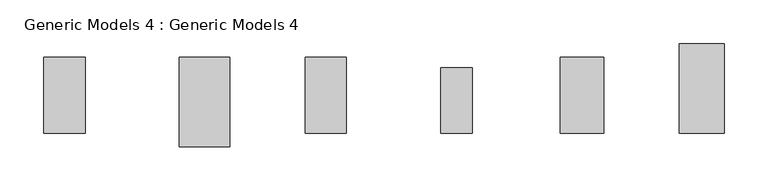
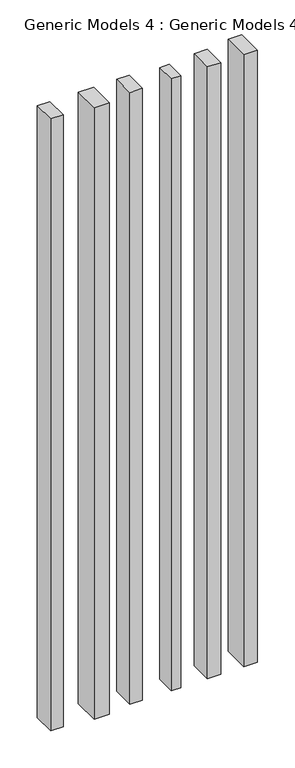
"""IFC4 building model written with IfcOpenShell, lengths in millimetres: proxy geometry, Generic Models 4 : Generic Models 4."""

from ifc_helpers import new_model, si_unit, frame, origin, place, context, project, spatial, polyline, outline, extrude, source, transform, mapped, element, save


def generic_models_4_generic_models_4_fedd3438(model_context):
    return source(origin(), model_context, "Body", "SweptSolid", [
        extrude(outline(polyline([(-9124.5906859, -16027.7337337), (-9073.7906859, -16027.7337337), (-9073.7906859, -16129.3337337), (-9124.5906859, -16129.3337337), (-9124.5906859, -16027.7337337)])), frame((0.0, 0.0, 3978.3517748), z_axis=(0.0, 0.0, 1.0), x_axis=(1.0, 0.0, 0.0)), (0.0, 0.0, 1.0), 2422.4482252),
        extrude(outline(polyline([(-9260.4094994, -16129.3337337), (-9260.4094994, -16043.033522), (-9210.5287858, -16043.033522), (-9210.5287858, -16129.3337337), (-9260.4094994, -16129.3337337)])), frame((0.0, 0.0, 3978.3517748), z_axis=(0.0, 0.0, 1.0), x_axis=(1.0, 0.0, 0.0)), (0.0, 0.0, 1.0), 2422.4482252),
        extrude(outline(polyline([(-9396.1073494, -16055.0872466), (-9360.4707697, -16055.0872466), (-9360.4707697, -16129.3337337), (-9396.1073494, -16129.3337337), (-9396.1073494, -16055.0872466)])), frame((0.0, 0.0, 3978.3517748), z_axis=(0.0, 0.0, 1.0), x_axis=(1.0, 0.0, 0.0)), (0.0, 0.0, 1.0), 2422.4482252),
        extrude(outline(polyline([(-9550.6380893, -16129.3337337), (-9550.6380893, -16043.033522), (-9503.708884, -16043.033522), (-9503.708884, -16129.3337337), (-9550.6380893, -16129.3337337)])), frame((0.0, 0.0, 3978.3517748), z_axis=(0.0, 0.0, 1.0), x_axis=(1.0, 0.0, 0.0)), (0.0, 0.0, 1.0), 2422.4482252),
        extrude(outline(polyline([(-9693.6024351, -16043.033522), (-9636.4524351, -16043.033522), (-9636.4524351, -16144.633522), (-9693.6024351, -16144.633522), (-9693.6024351, -16043.033522)])), frame((0.0, 0.0, 3978.3517748), z_axis=(0.0, 0.0, 1.0), x_axis=(1.0, 0.0, 0.0)), (0.0, 0.0, 1.0), 2422.4482252),
        extrude(outline(polyline([(-9847.8329873, -16129.3337337), (-9847.8329873, -16043.033522), (-9801.0960651, -16043.033522), (-9801.0960651, -16129.3337337), (-9847.8329873, -16129.3337337)])), frame((0.0, 0.0, 3978.3517748), z_axis=(0.0, 0.0, 1.0), x_axis=(1.0, 0.0, 0.0)), (0.0, 0.0, 1.0), 2422.4482252),
    ])


if __name__ == "__main__":
    model = new_model("IFC4")
    model_context = context("Model", 3, world=origin())
    ifc_project = project(units=[si_unit("LENGTHUNIT", "METRE", prefix="MILLI")], contexts=[model_context])
    site = spatial("IfcSite", under=ifc_project)
    building = spatial("IfcBuilding", under=site)
    placement = place(None, origin())
    generic_models_4_generic_models_4_shape = generic_models_4_generic_models_4_fedd3438(model_context)
    element("IfcBuildingElementProxy", 1, Name="Generic Models 4 : Generic Models 4", ObjectType="Generic Models 4 : Generic Models 4", at=placement, inside=building, context=model_context, shape_type="MappedRepresentation", body=[
        mapped(generic_models_4_generic_models_4_shape, transform((0.0, 0.0, 0.0), x_axis=(1.0, 0.0, 0.0), y_axis=(0.0, 1.0, 0.0), z_axis=(0.0, 0.0, 1.0))),
    ])
    save(model, "model.ifc")
